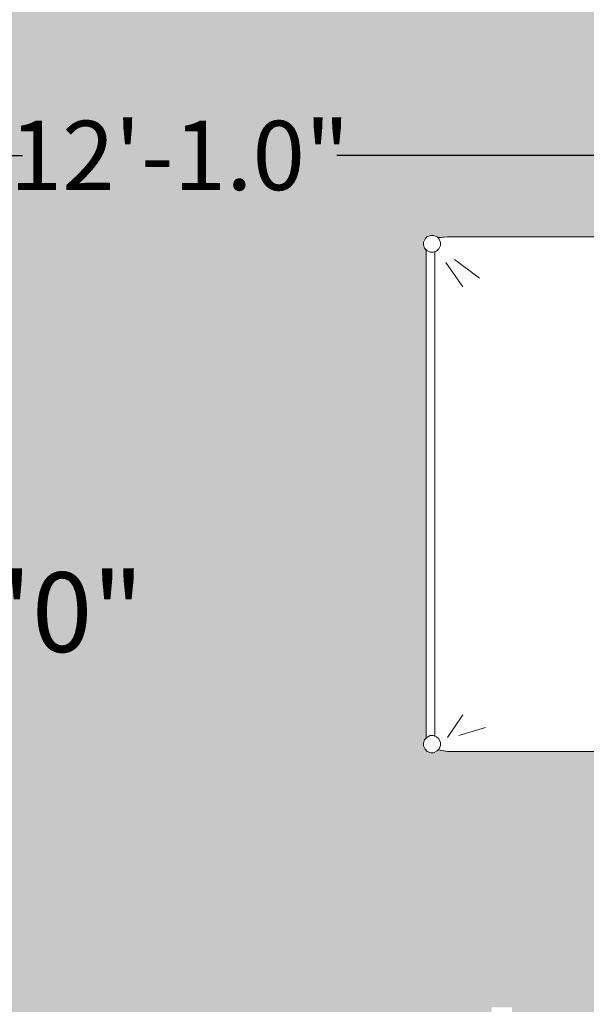
# Model space of a CAD drawing. Units: inches. Extents: x 528 to 2620, y -1066 to 798.
# Tile 8 of 41: x 688 to 737, y 620 to 705. Entities that reach past the tile are written whole.
import ezdxf

# ---------------------------------------------------------------- set-up
doc = ezdxf.new("R2010")
doc.units = ezdxf.units.IN
doc.header["$MEASUREMENT"] = 0
for name, color, linetype, lineweight in [('A-ANNO-DIMS', 2, 'Continuous', 18), ('A-AREA-IDEN', 7, 'Continuous', 18), ('A-FURN', 30, 'Continuous', 18), ('A-WALL-PATT', 8, 'Continuous', 13)]:
    doc.layers.add(name, color=color, linetype=linetype, lineweight=lineweight)
doc.styles.get("Standard").update_dxf_attribs({"font": 'arial.ttf'})
doc.dimstyles.get("Standard").update_dxf_attribs({"dimtxt": 6, "dimasz": 2, "dimexe": 0.18, "dimexo": 0.0625, "dimgap": 0.09, "dimtad": 0, "dimtih": 1, "dimtoh": 1, "dimdec": 1, "dimzin": 0, "dimdsep": 46, "dimlunit": 3, "dimtxsty": 'Standard', "dimblk": 'ARCHTICK', "dimcen": 0.09, "dimadec": 0, "dimazin": 0, "dimtfac": 1, "dimtdec": 1, "dimtofl": 0, "dimtmove": 0, "dimatfit": 3, "dimfxl": 1, "dimtolj": 1, "dimtzin": 0, "dimarcsym": 0})

# ---------------------------------------------------------------- blocks, each defined once
blk = doc.blocks.new('d-bed-3')
at = {"color": 0, "linetype": 'ByBlock'}
for p, q in [((0, 0), (0, -0.5)), ((0.7, 0), (0, 0)), ((0.7, -0.5), (0.7, 0)), ((0.7817, -0.0054), (0.7857, 0.0078)), ((0.7817, -0.0054), (0.7857, 0.0078)), ((0.7857, 0.0078), (0.7968, 0.0166)), ((0.7857, 0.0078), (0.7968, 0.0166)), ((0.7968, 0.0166), (0.8078, 0.0211)), ((0.7968, 0.0166), (0.8078, 0.0211)), ((0.8078, 0.0211), (0.8209, 0.0211)), ((0.8078, 0.0211), (0.8209, 0.0211)), ((0.8209, 0.0211), (0.8349, 0.0144)), ((0.8209, 0.0211), (0.8349, 0.0144)), ((0.8349, 0.0144), (0.8409, 0.0078)), ((0.8349, 0.0144), (0.8429, 0.0056)), ((0.8389, 0.0078), (2.7305, 0.0078)), ((0.8409, 0.0078), (2.7305, 0.0078)), ((0.8429, 0.0056), (0.848, -0.0077)), ((2.7234, -0.0077), (2.7284, 0.0056)), ((2.7284, 0.0056), (2.7365, 0.0144)), ((2.7305, 0.0078), (2.7365, 0.0144)), ((2.7365, 0.0144), (2.7505, 0.0211)), ((2.7365, 0.0144), (2.7505, 0.0211)), ((2.7505, 0.0211), (2.7636, 0.0211)), ((2.7505, 0.0211), (2.7636, 0.0211)), ((2.7636, 0.0211), (2.7746, 0.0166)), ((2.7636, 0.0211), (2.7746, 0.0166)), ((2.7746, 0.0166), (2.7857, 0.0078)), ((2.7746, 0.0166), (2.7857, 0.0078)), ((2.7857, 0.0078), (2.7897, -0.0054)), ((2.7857, 0.0078), (2.7897, -0.0054)), ((2.8714, -0.5), (2.8714, 0)), ((2.8714, 0), (3.5714, 0)), ((3.5714, 0), (3.5714, -0.5)), ((0.7817, -0.0187), (0.7817, -0.0054)), ((0.7817, -0.0187), (0.7817, -0.0054)), ((0.7857, -0.0297), (0.7817, -0.0187)), ((0.7857, -0.0297), (0.7817, -0.0187)), ((0.7857, -2.0939), (0.7857, -0.0297)), ((0.7948, -0.0408), (0.7857, -0.0297)), ((0.7857, -0.032), (0.7857, -2.0939)), ((0.8409, -0.032), (0.8319, -0.0408)), ((0.848, -0.0209), (0.8409, -0.032)), ((0.848, -0.0077), (0.848, -0.0209)), ((2.7234, -0.0209), (2.7234, -0.0077)), ((2.7305, -0.032), (2.7234, -0.0209)), ((2.7395, -0.0408), (2.7305, -0.032)), ((2.7857, -0.0297), (2.7766, -0.0408)), ((2.7857, -0.0297), (2.7766, -0.0408)), ((2.7897, -0.0187), (2.7857, -0.0297)), ((2.7897, -0.0187), (2.7857, -0.0297)), ((2.7897, -0.0054), (2.7897, -0.0187)), ((2.7897, -0.0054), (2.7897, -0.0187)), ((0.05, -0.05), (0.05, -0.45)), ((0.65, -0.05), (0.05, -0.05)), ((0.35, -0.0576), (0.35, -0.4424)), ((0.65, -0.45), (0.65, -0.05)), ((0.8058, -0.0452), (0.7948, -0.0408)), ((0.8188, -0.0452), (0.8058, -0.0452)), ((0.8319, -0.0408), (0.8188, -0.0452)), ((2.7525, -0.0452), (0.8188, -0.0452)), ((2.7525, -0.0452), (2.7395, -0.0408)), ((2.7656, -0.0452), (2.7525, -0.0452)), ((2.7766, -0.0408), (2.7656, -0.0452)), ((2.7766, -0.0408), (2.7656, -0.0452)), ((2.7656, -0.0452), (2.7857, -0.0452)), ((2.7857, -0.0452), (2.7656, -0.0452)), ((2.7857, -2.0939), (2.7857, -0.0452)), ((2.9214, -0.45), (2.9214, -0.05)), ((2.9214, -0.05), (3.5214, -0.05)), ((3.2214, -0.0576), (3.2214, -0.4424)), ((3.5214, -0.05), (3.5214, -0.45)), ((0.8781, -0.1325), (0.8911, -0.1059)), ((0.8911, -0.1059), (0.9182, -0.1082)), ((0.9182, -0.1082), (0.9443, -0.1148)), ((1.0317, -0.117), (1.0588, -0.1082)), ((1.0588, -0.1082), (1.0849, -0.1059)), ((1.0849, -0.1059), (1.113, -0.1104)), ((1.113, -0.1104), (1.1401, -0.117)), ((1.2295, -0.117), (1.2566, -0.1082)), ((1.2566, -0.1082), (1.2827, -0.1059)), ((1.2827, -0.1059), (1.3108, -0.1104)), ((1.3108, -0.1104), (1.3379, -0.117)), ((1.4253, -0.117), (1.4514, -0.1082)), ((1.4514, -0.1082), (1.4805, -0.1059)), ((1.4805, -0.1059), (1.5086, -0.1104)), ((1.5086, -0.1104), (1.5357, -0.117)), ((1.623, -0.1148), (1.6471, -0.1082)), ((1.6471, -0.1082), (1.6763, -0.1059)), ((1.6763, -0.1059), (1.7084, -0.1059)), ((1.7084, -0.1059), (1.7194, -0.1325)), ((1.8489, -0.1302), (1.863, -0.1059)), ((1.863, -0.1059), (1.8951, -0.1059)), ((1.8951, -0.1059), (1.9222, -0.1059)), ((1.9222, -0.1059), (1.9483, -0.1148)), ((2.0357, -0.1148), (2.0628, -0.1082)), ((2.0628, -0.1082), (2.0909, -0.1059)), ((2.0909, -0.1059), (2.117, -0.1082)), ((2.117, -0.1082), (2.1441, -0.1148)), ((2.2335, -0.1148), (2.2606, -0.1082)), ((2.2606, -0.1082), (2.2867, -0.1059)), ((2.2867, -0.1059), (2.3148, -0.1082)), ((2.3148, -0.1082), (2.3419, -0.1148)), ((2.4293, -0.1148), (2.4554, -0.1082)), ((2.4554, -0.1082), (2.4845, -0.1059)), ((2.4845, -0.1059), (2.5126, -0.1082)), ((2.5126, -0.1082), (2.5397, -0.1148)), ((2.627, -0.1148), (2.6511, -0.1059)), ((2.6511, -0.1059), (2.6803, -0.1059)), ((2.6803, -0.1059), (2.6913, -0.1302)), ((0.8721, -0.159), (0.8781, -0.1325)), ((0.9072, -0.5753), (0.9072, -0.1391)), ((0.9072, -0.1391), (1.6763, -0.1391)), ((0.9293, -0.1435), (0.9775, -0.1612)), ((0.9443, -0.1148), (0.9684, -0.128)), ((0.9684, -0.128), (1.0056, -0.128)), ((1.0056, -0.128), (1.0317, -0.117)), ((1.1401, -0.117), (1.1662, -0.128)), ((1.1662, -0.128), (1.2034, -0.128)), ((1.2034, -0.128), (1.2295, -0.117)), ((1.3379, -0.117), (1.362, -0.128)), ((1.362, -0.128), (1.4012, -0.128)), ((1.4012, -0.128), (1.4253, -0.117)), ((1.5357, -0.117), (1.5598, -0.128)), ((1.5598, -0.128), (1.5989, -0.128)), ((1.5989, -0.128), (1.623, -0.1148)), ((1.6471, -0.1501), (1.5989, -0.1656)), ((1.6763, -0.1391), (1.6763, -0.4936)), ((1.7194, -0.1325), (1.7265, -0.159)), ((1.8429, -0.159), (1.8489, -0.1302)), ((2.6622, -0.1369), (1.8931, -0.1369)), ((1.8931, -0.1369), (1.8931, -0.5046)), ((1.9222, -0.1479), (1.9704, -0.1656)), ((1.9483, -0.1148), (1.9724, -0.128)), ((1.9724, -0.128), (2.0096, -0.128)), ((2.0096, -0.128), (2.0357, -0.1148)), ((2.1441, -0.1148), (2.1702, -0.128)), ((2.1702, -0.128), (2.2074, -0.128)), ((2.2074, -0.128), (2.2335, -0.1148)), ((2.3419, -0.1148), (2.366, -0.128)), ((2.366, -0.128), (2.4052, -0.128)), ((2.4052, -0.128), (2.4293, -0.1148)), ((2.5397, -0.1148), (2.5638, -0.128)), ((2.5638, -0.128), (2.6029, -0.128)), ((2.6401, -0.1435), (2.5919, -0.159)), ((2.6029, -0.128), (2.627, -0.1148)), ((2.6622, -0.5753), (2.6622, -0.1369)), ((2.6913, -0.1302), (2.6973, -0.159)), ((0.8741, -0.1866), (0.8721, -0.159)), ((0.8831, -0.2131), (0.8741, -0.1866)), ((0.9223, -0.1612), (0.9333, -0.2042)), ((1.6542, -0.1656), (1.6431, -0.2087)), ((1.7265, -0.1866), (1.7174, -0.2131)), ((1.7265, -0.159), (1.7265, -0.1866)), ((1.8449, -0.1866), (1.8429, -0.159)), ((1.854, -0.2131), (1.8449, -0.1866)), ((1.9152, -0.1656), (1.9263, -0.2087)), ((2.6471, -0.159), (2.6361, -0.202)), ((2.6973, -0.1866), (2.6883, -0.2131)), ((2.6973, -0.159), (2.6973, -0.1866)), ((0.8962, -0.2374), (0.8831, -0.2131)), ((1.7174, -0.2131), (1.7024, -0.2374)), ((1.867, -0.2374), (1.854, -0.2131)), ((2.6883, -0.2131), (2.6732, -0.2374)), ((0.1576, -0.25), (0.5424, -0.25)), ((0.8962, -0.2992), (0.8962, -0.2374)), ((1.7024, -0.2374), (1.7024, -0.2992)), ((1.867, -0.297), (1.867, -0.2374)), ((2.6732, -0.2374), (2.6732, -0.297)), ((3.4138, -0.25), (3.029, -0.25)), ((0.8831, -0.3235), (0.8962, -0.2992)), ((1.7024, -0.2992), (1.7174, -0.3235)), ((1.854, -0.3213), (1.867, -0.297)), ((2.6732, -0.297), (2.6883, -0.3213)), ((0.8761, -0.3489), (0.8831, -0.3235)), ((1.0538, -0.6294), (1.362, -0.3081)), ((1.362, -0.3081), (1.619, -0.5532)), ((1.7174, -0.3235), (1.7244, -0.3489)), ((1.8469, -0.3489), (1.854, -0.3213)), ((2.2074, -0.3081), (1.9483, -0.5532)), ((2.5146, -0.6294), (2.2074, -0.3081)), ((2.6883, -0.3213), (2.6953, -0.3489)), ((0.8761, -0.3776), (0.8761, -0.3489)), ((0.8831, -0.4041), (0.8761, -0.3776)), ((1.3289, -0.3511), (1.3068, -0.3909)), ((1.4052, -0.3467), (1.4122, -0.4019)), ((1.7244, -0.3776), (1.7174, -0.4041)), ((1.7244, -0.3489), (1.7244, -0.3776)), ((1.8469, -0.3754), (1.8469, -0.3489)), ((1.854, -0.4041), (1.8469, -0.3754)), ((2.1632, -0.3445), (2.1572, -0.3997)), ((2.2405, -0.3511), (2.2626, -0.3887)), ((2.6953, -0.3754), (2.6883, -0.4041)), ((2.6953, -0.3489), (2.6953, -0.3754)), ((0.8962, -0.4284), (0.8831, -0.4041)), ((1.3068, -0.3909), (1.3349, -0.4174)), ((1.4122, -0.4019), (1.3901, -0.4284)), ((1.4674, -0.7134), (1.7746, -0.3909)), ((1.7174, -0.4041), (1.7024, -0.4284)), ((1.7746, -0.3909), (2.0979, -0.6979)), ((1.867, -0.4284), (1.854, -0.4041)), ((2.1572, -0.3997), (2.1793, -0.4284)), ((2.2626, -0.3887), (2.2335, -0.4174)), ((2.6883, -0.4041), (2.6732, -0.4284)), ((0.05, -0.45), (0.65, -0.45)), ((0.8962, -0.4781), (0.8962, -0.4284)), ((1.5006, -0.4505), (1.4604, -0.4715)), ((1.7024, -0.4284), (1.7024, -0.4649)), ((1.7415, -0.4351), (1.7194, -0.4737)), ((1.8188, -0.4306), (1.8228, -0.4848)), ((1.867, -0.4781), (1.867, -0.4284)), ((2.0688, -0.4505), (2.109, -0.4715)), ((2.6732, -0.4284), (2.6732, -0.4759)), ((3.5214, -0.45), (2.9214, -0.45)), ((0.8831, -0.5024), (0.8962, -0.4781)), ((1.2255, -0.4715), (1.2626, -0.5223)), ((1.5327, -0.4715), (1.4674, -0.5267)), ((1.7194, -0.4737), (1.7485, -0.5002)), ((1.8228, -0.4848), (1.8008, -0.5113)), ((2.0357, -0.4715), (2.102, -0.5267)), ((2.3439, -0.4715), (2.3068, -0.5201)), ((2.6732, -0.4759), (2.6883, -0.5002)), ((0, -0.5), (0.7, -0.5)), ((0.8721, -0.5576), (0.8741, -0.5289)), ((0.8741, -0.5289), (0.8831, -0.5024)), ((0.9223, -0.5532), (0.9333, -0.5113)), ((1.9112, -0.5333), (1.874, -0.5554)), ((2.6471, -0.5532), (2.6361, -0.5091)), ((2.6883, -0.5002), (2.6973, -0.5267)), ((2.6973, -0.5267), (2.6973, -0.5554)), ((3.5714, -0.5), (2.8714, -0.5)), ((0.8781, -0.5841), (0.8721, -0.5576)), ((0.9293, -0.5709), (0.9775, -0.5532)), ((1.2957, -0.5819), (1.2737, -0.5488)), ((1.3399, -0.5643), (1.3399, -0.5488)), ((1.357, -0.625), (1.3399, -0.5643)), ((1.5989, -0.5488), (1.614, -0.5554)), ((1.6381, -0.5554), (1.6763, -0.6051)), ((1.9443, -0.5554), (1.8781, -0.6096)), ((1.9704, -0.5466), (1.9503, -0.5554)), ((2.2124, -0.6228), (2.2295, -0.5643)), ((2.2295, -0.5643), (2.2295, -0.5466)), ((2.2736, -0.5797), (2.2957, -0.5466)), ((2.6401, -0.5687), (2.5919, -0.5532)), ((2.6973, -0.5554), (2.6913, -0.5841)), ((0.8911, -0.6096), (0.8781, -0.5841)), ((0.9182, -0.6073), (0.8911, -0.6096)), ((1.109, -0.5753), (0.9072, -0.5753)), ((0.9443, -0.6007), (0.9182, -0.6073)), ((0.9684, -0.5886), (0.9443, -0.6007)), ((1.0056, -0.5886), (0.9684, -0.5886)), ((1.0317, -0.5996), (1.0056, -0.5886)), ((1.0588, -0.6073), (1.0317, -0.5996)), ((1.0759, -0.6096), (1.0588, -0.6073)), ((1.105, -0.5864), (1.1271, -0.5864)), ((1.1271, -0.5864), (1.1482, -0.5974)), ((1.1482, -0.5974), (1.1311, -0.5864)), ((1.1311, -0.5864), (1.1592, -0.593)), ((1.3459, -0.625), (1.2957, -0.5819)), ((1.5658, -0.5753), (1.5377, -0.5864)), ((1.5969, -0.5753), (1.5658, -0.5753)), ((1.9684, -0.5753), (2.0036, -0.5753)), ((2.0036, -0.5753), (2.0317, -0.5864)), ((2.1963, -0.6294), (2.124, -0.6118)), ((2.2224, -0.6228), (2.2736, -0.5797)), ((2.4383, -0.5864), (2.4092, -0.5908)), ((2.4423, -0.5864), (2.4202, -0.5974)), ((2.4202, -0.5974), (2.4383, -0.5864)), ((2.4644, -0.5864), (2.4423, -0.5864)), ((2.4604, -0.5753), (2.6622, -0.5753)), ((2.5126, -0.6051), (2.4955, -0.6073)), ((2.5397, -0.5996), (2.5126, -0.6051)), ((2.5638, -0.5864), (2.5397, -0.5996)), ((2.6029, -0.5864), (2.5638, -0.5864)), ((2.627, -0.5996), (2.6029, -0.5864)), ((2.6511, -0.6073), (2.627, -0.5996)), ((2.6803, -0.6073), (2.6511, -0.6073)), ((2.6913, -0.5841), (2.6803, -0.6073)), ((1.3791, -0.9365), (1.0538, -0.6294)), ((1.3138, -0.6626), (1.351, -0.6361)), ((1.368, -0.6626), (1.357, -0.625)), ((1.3731, -0.6294), (1.4453, -0.614)), ((1.3791, -0.6471), (1.4453, -0.6913)), ((1.7084, -0.6648), (1.6873, -0.6316)), ((1.7526, -0.6493), (1.7526, -0.6316)), ((1.7706, -0.7089), (1.7526, -0.6493)), ((2.0387, -0.6427), (2.0427, -0.6405)), ((2.1903, -0.6449), (2.124, -0.6891)), ((2.1903, -0.9365), (2.5146, -0.6294)), ((2.2013, -0.6626), (2.2124, -0.6228)), ((2.2556, -0.6626), (2.2184, -0.6338)), ((1.105, -0.6692), (1.1421, -0.6846)), ((1.1421, -0.6846), (1.1642, -0.6736)), ((1.1642, -0.6736), (1.1753, -0.6692)), ((1.3731, -0.6692), (1.3841, -0.7067)), ((1.7596, -0.7089), (1.7084, -0.6648)), ((1.9765, -0.6604), (1.9503, -0.6714)), ((2.0166, -0.6604), (1.9765, -0.6604)), ((2.0387, -0.6714), (2.0166, -0.6604)), ((2.1963, -0.667), (2.1853, -0.7067)), ((2.4052, -0.6736), (2.3941, -0.667)), ((2.4272, -0.6846), (2.4052, -0.6736)), ((2.4644, -0.667), (2.4272, -0.6846)), ((1.2255, -0.7785), (1.2737, -0.7244)), ((1.4674, -0.7134), (1.4604, -0.7067)), ((1.7897, -1.0193), (1.4674, -0.7134)), ((1.7265, -0.7454), (1.7636, -0.72)), ((1.7817, -0.7454), (1.7706, -0.7089)), ((1.7857, -0.7134), (1.856, -0.6979)), ((2.0979, -0.6979), (1.7897, -1.0193)), ((1.9724, -0.741), (1.9393, -0.7244)), ((2.0538, -0.7609), (2.109, -0.7067)), ((2.3439, -0.7763), (2.2957, -0.7222)), ((1.5548, -0.7675), (1.5397, -0.7631)), ((1.5548, -0.7675), (1.5769, -0.7564)), ((1.5769, -0.7564), (1.5879, -0.752)), ((1.7857, -0.752), (1.7967, -0.7896)), ((1.7897, -0.731), (1.856, -0.7741)), ((2.0096, -0.741), (1.9724, -0.741)), ((2.0497, -0.731), (2.0096, -0.741)), ((1.3791, -0.9365), (1.5357, -0.7763)), ((1.9283, -0.8448), (1.874, -0.7896)), ((2.1903, -0.9365), (2.0277, -0.7697)), ((0.7857, -0.9607), (1.2295, -0.8072)), ((0.9504, -1.2611), (1.5708, -0.8183)), ((1.3178, -0.8382), (1.3239, -0.8117)), ((1.3178, -0.8602), (1.3178, -0.8382)), ((1.4052, -0.8337), (1.4012, -0.8337)), ((1.4052, -0.8768), (1.4052, -0.8337)), ((1.6381, -0.8625), (1.6873, -0.8072)), ((2.618, -1.2611), (1.9855, -0.8161)), ((2.1632, -0.8757), (2.1632, -0.8315)), ((2.1632, -0.8315), (2.1682, -0.8315)), ((2.2515, -0.8382), (2.2445, -0.8094)), ((2.2515, -0.8602), (2.2515, -0.8382)), ((2.7827, -0.9607), (2.3278, -0.8072)), ((1.3349, -0.8879), (1.3178, -0.8602)), ((1.3901, -0.8989), (1.4052, -0.8768)), ((2.1793, -0.8967), (2.1632, -0.8757)), ((2.2335, -0.8856), (2.2515, -0.8602)), ((0.8781, -1.2059), (1.3349, -0.9055)), ((1.7305, -0.921), (1.7375, -0.8945)), ((1.8188, -0.9166), (1.8118, -0.9166)), ((1.8188, -0.9607), (1.8188, -0.9166)), ((2.6913, -1.2059), (2.2254, -0.9055)), ((1.7305, -0.9431), (1.7305, -0.921)), ((1.7485, -0.9718), (1.7305, -0.9431)), ((0.8128, -1.0115), (0.7857, -0.9607)), ((1.8008, -0.9828), (1.8188, -0.9607)), ((2.7676, -0.9895), (2.7455, -1.0259)), ((2.7786, -0.9828), (2.7676, -0.9895)), ((2.7827, -0.9607), (2.7786, -0.9828)), ((0.8128, -1.0325), (0.8128, -1.0115)), ((0.8239, -1.0414), (0.8128, -1.0325)), ((2.7455, -1.0259), (2.7234, -1.0811)), ((0.8299, -1.0635), (0.8239, -1.0414)), ((0.8349, -1.0745), (0.8299, -1.0635)), ((0.845, -1.1032), (0.8349, -1.0745)), ((0.852, -1.1187), (0.845, -1.1032)), ((2.7234, -1.1076), (2.7174, -1.1187)), ((2.7234, -1.0811), (2.7234, -1.1076)), ((0.852, -1.1363), (0.852, -1.1187)), ((0.863, -1.1617), (0.852, -1.1363)), ((2.7124, -1.1253), (2.6953, -1.1617)), ((2.7174, -1.1187), (2.7124, -1.1253)), ((0.867, -1.1905), (0.863, -1.1617)), ((0.9223, -1.2015), (0.9112, -1.1838)), ((2.6582, -1.1838), (2.6471, -1.2015)), ((2.6953, -1.1617), (2.6913, -1.2059)), ((0.8741, -1.1949), (0.867, -1.1905)), ((0.8781, -1.2059), (0.8741, -1.1949)), ((0.9293, -1.2059), (0.9223, -1.2015)), ((0.9403, -1.2236), (0.9293, -1.2059)), ((0.9443, -1.2391), (0.9403, -1.2236)), ((2.6361, -1.2236), (2.625, -1.2391)), ((2.6471, -1.2015), (2.6361, -1.2236)), ((0.9504, -1.2611), (0.9443, -1.2391)), ((2.625, -1.2391), (2.618, -1.2611)), ((2.7234, -2.0497), (2.6913, -1.947)), ((0.8741, -2.0673), (0.9464, -1.9691)), ((0.8851, -2.1005), (0.9795, -2.0342)), ((2.7305, -2.0939), (2.6421, -2.0342)), ((0.7888, -2.1317), (0.7857, -2.0939)), ((0.7857, -2.0939), (0.7887, -2.1303)), ((2.7857, -2.0939), (2.7783, -2.1299)), ((2.7786, -2.1281), (2.7857, -2.0939)), ((0.7797, -2.148), (0.7857, -2.1347)), ((0.7797, -2.148), (0.7857, -2.1347)), ((0.7857, -2.1347), (0.7948, -2.1259)), ((0.7857, -2.1347), (0.7888, -2.1317)), ((0.7948, -2.1259), (0.8078, -2.1215)), ((0.8078, -2.1215), (0.8188, -2.1215)), ((0.8188, -2.1215), (0.8319, -2.1281)), ((0.8319, -2.1281), (0.8409, -2.1369)), ((0.8409, -2.1369), (0.845, -2.1502)), ((2.7284, -2.1369), (2.7234, -2.1502)), ((2.7365, -2.1281), (2.7284, -2.1369)), ((2.7505, -2.1215), (2.7365, -2.1281)), ((2.7616, -2.1215), (2.7505, -2.1215)), ((2.7746, -2.1259), (2.7616, -2.1215)), ((2.7827, -2.1347), (2.7746, -2.1259)), ((2.7783, -2.1299), (2.7827, -2.1347)), ((2.7827, -2.1347), (2.7897, -2.148)), ((2.7897, -2.148), (2.7827, -2.1347)), ((0.7797, -2.159), (0.7797, -2.148)), ((0.7797, -2.148), (0.7797, -2.159)), ((0.7837, -2.1723), (0.7797, -2.159)), ((0.7837, -2.1723), (0.7797, -2.159)), ((0.7927, -2.1811), (0.7837, -2.1723)), ((0.7927, -2.1811), (0.7837, -2.1723)), ((0.8389, -2.1745), (0.8299, -2.1833)), ((0.8367, -2.1767), (0.8299, -2.1833)), ((2.7327, -2.1767), (0.8367, -2.1767)), ((0.845, -2.1612), (0.8389, -2.1745)), ((0.8389, -2.1767), (2.7305, -2.1767)), ((2.7264, -2.1436), (0.845, -2.1436)), ((0.845, -2.1502), (0.845, -2.1612)), ((2.7234, -2.1502), (2.7234, -2.1612)), ((2.7234, -2.1612), (2.7305, -2.1745)), ((2.7305, -2.1745), (2.7395, -2.1833)), ((2.7395, -2.1833), (2.7327, -2.1767)), ((2.7857, -2.1723), (2.7766, -2.1811)), ((2.7766, -2.1811), (2.7857, -2.1723)), ((2.7897, -2.159), (2.7857, -2.1723)), ((2.7857, -2.1723), (2.7897, -2.159)), ((2.7897, -2.148), (2.7897, -2.159)), ((2.7897, -2.159), (2.7897, -2.148)), ((0.8058, -2.1877), (0.7927, -2.1811)), ((0.8058, -2.1877), (0.7927, -2.1811)), ((0.8168, -2.1877), (0.8058, -2.1877)), ((0.8168, -2.1877), (0.8058, -2.1877)), ((0.8299, -2.1833), (0.8168, -2.1877)), ((0.8299, -2.1833), (0.8168, -2.1877)), ((2.7525, -2.1877), (2.7395, -2.1833)), ((2.7395, -2.1833), (2.7525, -2.1877)), ((2.7636, -2.1877), (2.7525, -2.1877)), ((2.7525, -2.1877), (2.7636, -2.1877)), ((2.7766, -2.1811), (2.7636, -2.1877)), ((2.7636, -2.1877), (2.7766, -2.1811))]:
    blk.add_line(p, q, dxfattribs=at)
blk.add_ellipse((0.35, -0.25), major_axis=(-0.1007, 0.1007), ratio=1, dxfattribs=at)
at = {"color": 0, "linetype": 'ByBlock', "extrusion": (0, 0, -1)}
blk.add_ellipse((3.2214, -0.25), major_axis=(0.1007, 0.1007), ratio=1, dxfattribs=at)
blk = doc.blocks.new('_ArchTick')
at = {"color": 0, "linetype": 'ByBlock', "const_width": 0.15}
blk.add_lwpolyline([(-0.5, -0.5), (0.5, 0.5)], dxfattribs=at)
blk = doc.blocks.new('*D25')
at = {"layer": 'A-ANNO-DIMS', "color": 0, "lineweight": -2, "transparency": 16777216}
for p, q in [((629.059, 693.763), (629.059, 693.001)), ((774.059, 693.763), (774.059, 693.001)), ((629.059, 693.181), (687.951, 693.181)), ((774.059, 693.181), (715.168, 693.181))]:
    blk.add_line(p, q, dxfattribs=at)
at = {"layer": 'Defpoints', "color": 0, "transparency": 16777216}
for p in [(629.059, 693.826), (774.059, 693.826), (774.059, 693.181)]:
    blk.add_point(p, dxfattribs=at)
at = {"layer": 'A-ANNO-DIMS', "color": 0, "lineweight": -2, "transparency": 16777216, "xscale": 2, "yscale": 2, "zscale": 2, "rotation": 180}
blk.add_blockref('_ArchTick', (629.059, 693.181), dxfattribs=at)
at = {"layer": 'A-ANNO-DIMS', "color": 0, "lineweight": -2, "transparency": 16777216, "xscale": 2, "yscale": 2, "zscale": 2}
blk.add_blockref('_ArchTick', (774.059, 693.181), dxfattribs=at)
at = {"layer": 'A-ANNO-DIMS', "color": 0, "transparency": 16777216, "insert": (701.559, 693.181), "char_height": 6, "attachment_point": 5}
blk.add_mtext('\\A1;12\'-1.0"', dxfattribs=at)

msp = doc.modelspace()

# ---------------------------------------------------------------- hatches: boundary and pattern name
at = {"layer": 'A-WALL-PATT', "transparency": 33554687}
h = msp.add_hatch(color=256, dxfattribs=at)
h.dxf.hatch_style = 1
h.paths.add_polyline_path([(861.059, 273.922), (817.059, 273.922), (817.059, 272.922), (861.059, 272.922)])
h.paths.add_polyline_path([(817.059, 277.922), (815.059, 277.922), (815.059, 268.922), (817.059, 268.922)])
h.paths.add_polyline_path([(908.059, 397.922), (899.059, 397.922), (899.059, 395.922), (908.059, 395.922)])
h.paths.add_polyline_path([(908.059, 443.922), (899.059, 443.922), (899.059, 441.922), (908.059, 441.922)])
h.paths.add_polyline_path([(904.059, 441.922), (903.059, 441.922), (903.059, 397.922), (904.059, 397.922)])
h.paths.add_polyline_path([(625.059, 561.422), (624.059, 561.422), (624.059, 537.422), (625.059, 537.422)])
h.paths.add_polyline_path([(648.747, 334.444), (720.045, 334.444), (720.045, 344.998), (648.747, 344.998)], flags=9)
h.paths.add_polyline_path([(819.733, 323.153), (880.328, 323.153), (880.328, 333.708), (819.733, 333.708)], flags=9)
h.paths.add_polyline_path([(779.898, 680.607), (821.764, 680.607), (821.764, 691.169), (779.898, 691.169)], flags=9)
h.paths.add_polyline_path([(779.876, 692.362), (817.138, 692.362), (817.138, 703.058), (779.876, 703.058)], flags=9)
h.paths.add_polyline_path([(799.994, 453.884), (860.589, 453.884), (860.589, 464.439), (799.994, 464.439)], flags=9)
h.paths.add_polyline_path([(650.866, 539.397), (708.781, 539.397), (708.781, 549.952), (650.866, 549.952)], flags=9)
h.paths.add_polyline_path([(788.504, 612.01), (849.099, 612.01), (849.099, 622.565), (788.504, 622.565)], flags=9)
h.paths.add_polyline_path([(639.539, 648.31), (700.134, 648.31), (700.134, 658.865), (639.539, 658.865)], flags=9)
h.paths.add_polyline_path([(648.913, 346.09), (747.706, 346.09), (747.706, 356.778), (648.913, 356.778)], flags=9)
h.paths.add_polyline_path([(676.857, 450.66), (746.735, 450.66), (746.735, 461.355), (676.857, 461.355)], flags=9)
h.paths.add_polyline_path([(819.711, 334.947), (865.526, 334.947), (865.526, 345.636), (819.711, 345.636)], flags=9)
h.paths.add_polyline_path([(806.298, 467.745), (874.047, 467.745), (874.047, 478.441), (806.298, 478.441)], flags=9)
h.paths.add_polyline_path([(653.235, 552.284), (690.497, 552.284), (690.497, 562.979), (653.235, 562.979)], flags=9)
h.paths.add_polyline_path([(789.903, 623.407), (843.208, 623.407), (843.208, 634.103), (789.903, 634.103)], flags=9)
h.paths.add_polyline_path([(639.773, 662.103), (693.077, 662.103), (693.077, 672.798), (639.773, 672.798)], flags=9)
h.paths.add_polyline_path([(801.587, 242.914), (846.334, 242.914), (846.334, 253.603), (801.587, 253.603)], flags=9)
h.paths.add_polyline_path([(925.362, 593.982), (925.362, 674.057), (914.673, 674.057), (914.673, 593.982)], flags=9)
h.paths.add_polyline_path([(612.559, 593.982), (612.559, 674.057), (601.871, 674.057), (601.871, 593.982)], flags=9)
h.paths.add_polyline_path([(723.31, 726.564), (803.385, 726.564), (803.385, 737.252), (723.31, 737.252)], flags=9)
at = {"layer": 'A-WALL-PATT', "transparency": 33554590}
h = msp.add_hatch(color=256, dxfattribs=at)
h.dxf.hatch_style = 1
h.paths.add_polyline_path([(774.059, 709.922), (629.059, 709.922), (629.059, 577.922), (728.559, 577.922), (728.559, 579.422), (728.559, 619.422), (730.309, 619.422), (730.309, 619.384, -0.401453), (768.559, 579.422), (768.559, 577.922), (774.059, 577.922)])
h.paths.add_polyline_path([(723.896, 686.058), (723.968, 686.064), (723.828, 686.128)], flags=0)
h.paths.add_polyline_path([(722.785, 642.699), (722.893, 642.756), (722.893, 684.992), (722.647, 685.244), (722.647, 685.82), (723.079, 686.262), (723.533, 686.262), (723.968, 686.064), (724.739, 686.128), (770.696, 686.128), (770.78, 686.14), (771.126, 686.266), (771.694, 686.094), (771.94, 685.478), (771.67, 684.904), (771.582, 684.871), (771.582, 642.782), (771.878, 642.514), (771.878, 641.921), (771.511, 641.462), (770.855, 641.462), (770.401, 641.833), (770.401, 641.551), (724.739, 641.551), (723.991, 641.705), (723.443, 641.414), (722.879, 641.585), (722.597, 642.142)], flags=16)
h.paths.add_polyline_path([(723.994, 641.704), (723.994, 641.707), (723.991, 641.705)], flags=0)
h.paths.add_polyline_path([(722.893, 642.732), (722.893, 684.992), (722.647, 685.244), (722.647, 685.82), (723.079, 686.262), (723.287, 686.262), (722.991, 686.172), (722.794, 685.971), (722.647, 685.68), (722.647, 685.434), (722.745, 685.143), (722.942, 684.942), (723.238, 684.807), (723.484, 684.807), (723.779, 684.897), (723.976, 685.098), (724.174, 685.488), (724.124, 685.635), (724.124, 685.249), (723.631, 684.746), (723.631, 642.961), (724.124, 642.514), (724.124, 641.887), (723.656, 641.462), (723.079, 641.462), (722.647, 641.904), (722.647, 642.48)], flags=0)
h.paths.add_polyline_path([(722.647, 642.29), (722.647, 642.044), (722.794, 641.753), (723.079, 641.462), (723.287, 641.462), (722.879, 641.585), (722.597, 642.142)], flags=0)
h.paths.add_polyline_path([(770.745, 686.128), (770.58, 686.128), (770.551, 686.057)], flags=0)
h.paths.add_polyline_path([(743.299, 645.288), (753.227, 659.398), (748.69, 663.75), (753.234, 668.538), (743.299, 682.458), (743.791, 682.592), (744.136, 682.681), (744.53, 682.928), (744.628, 683.084), (745.017, 683.327), (744.53, 684.069), (744.776, 684.158), (744.874, 684.315), (745.514, 684.404), (746.081, 684.651), (746.474, 684.651), (746.819, 684.807), (747.459, 685.031), (747.705, 685.143), (748.198, 685.277), (748.394, 685.523), (748.862, 685.523), (749.994, 686.128), (753.488, 676.03), (757.379, 680.153), (757.791, 679.758), (758.044, 680.645), (758.29, 681.227), (758.29, 682.055), (758.019, 682.592), (757.871, 683.174), (757.822, 683.778), (758.388, 684.069), (758.979, 684.203), (759.619, 684.158), (760.21, 683.957), (760.751, 683.666), (761.859, 683.666), (762.401, 683.957), (762.991, 684.114), (763.631, 684.114), (764.198, 683.957), (764.739, 683.666), (766.118, 683.666), (766.659, 683.957), (767.25, 684.158), (767.865, 684.203), (768.456, 684.069), (769.047, 683.778), (768.998, 683.174), (768.85, 682.592), (768.554, 682.055), (768.554, 681.227), (768.801, 680.645), (769.092, 679.75), (768.948, 678.832), (768.801, 678.228), (768.554, 677.646), (768.554, 676.818), (768.801, 676.237), (769.092, 675.341), (768.948, 674.424), (768.801, 673.82), (768.554, 673.283), (768.554, 672.41), (768.801, 671.873), (768.998, 671.291), (769.047, 670.642), (768.948, 670.016), (768.801, 669.411), (768.554, 668.874), (768.554, 668.002), (768.974, 667.239), (769.047, 666.279), (769.047, 665.563), (768.456, 665.316), (767.865, 665.16), (767.25, 665.16), (766.659, 665.361), (766.118, 665.697), (764.739, 665.697), (763.945, 665.204), (762.991, 665.204), (762.401, 665.361), (761.859, 665.697), (761.005, 665.697), (762.696, 664.086), (760.741, 662.027), (761.859, 662.027), (762.401, 662.318), (763.342, 662.548), (764.247, 662.318), (764.788, 662.027), (766.118, 662.027), (766.659, 662.318), (767.25, 662.519), (767.865, 662.564), (768.505, 662.43), (769.047, 662.116), (769.047, 661.4), (769.047, 660.796), (768.85, 660.214), (768.554, 659.677), (768.554, 658.849), (768.85, 658.267), (768.998, 657.663), (769.069, 656.749), (768.85, 655.851), (768.554, 655.269), (768.554, 654.441), (768.85, 653.859), (769.069, 652.961), (768.998, 652.046), (768.85, 651.442), (768.554, 650.905), (768.554, 650.032), (768.85, 649.495), (768.998, 648.914), (769.047, 648.265), (768.998, 647.638), (768.85, 647.034), (768.554, 646.497), (768.554, 645.624), (768.85, 645.087), (769.047, 644.55), (769.047, 643.901), (768.505, 643.655), (767.865, 643.521), (767.25, 643.521), (766.659, 643.722), (766.118, 644.058), (764.788, 644.058), (764.247, 643.722), (763.342, 643.492), (762.401, 643.722), (761.859, 644.058), (760.801, 644.058), (760.259, 643.722), (759.668, 643.521), (759.028, 643.521), (758.388, 643.655), (757.871, 643.901), (757.871, 644.55), (758.044, 645.087), (758.339, 645.624), (758.339, 646.497), (758.044, 647.034), (757.921, 647.638), (757.866, 648.059), (757.379, 647.593), (753.422, 651.773), (749.994, 641.618), (749.502, 641.708), (749.354, 641.954), (748.542, 642.446), (747.311, 642.939), (746.652, 642.939), (746.327, 643.185), (745.514, 643.565), (744.53, 643.655), (745.011, 644.4), (744.628, 644.639), (744.136, 644.886), (743.791, 645.132)], flags=0)
h.paths.add_polyline_path([(755.656, 654.933), (756.542, 654.687), (757.527, 654.329), (756.641, 654.575)], flags=0)
h.paths.add_polyline_path([(758.339, 649.204), (758.339, 648.712), (758.585, 644.304), (758.585, 648.802)], flags=0)
h.paths.add_polyline_path([(758.339, 649.294), (758.093, 649.697), (758.359, 649.165)], flags=0)
h.paths.add_polyline_path([(755.656, 672.79), (756.493, 673.037), (757.358, 673.351), (757.353, 673.358), (756.641, 673.149)], flags=0)
h.paths.add_polyline_path([(760.264, 639.641), (771.408, 639.641), (771.408, 624.039), (760.264, 624.039)], flags=16)
h.paths.add_polyline_path([(761.378, 638.526), (770.294, 638.526), (770.294, 625.153), (761.378, 625.153)], flags=0)
edge = h.paths.add_edge_path(flags=0)
edge.add_ellipse((765.836, 631.84), major_axis=(-2.245, 2.245), ratio=1, start_angle=-45, end_angle=45, ccw=False)
edge.add_ellipse((765.836, 631.84), major_axis=(-2.245, 2.245), ratio=1, start_angle=-135, end_angle=-45, ccw=False)
edge.add_ellipse((765.836, 631.84), major_axis=(-2.245, 2.245), ratio=1, start_angle=135, end_angle=-135, ccw=False)
edge.add_ellipse((765.836, 631.84), major_axis=(-2.245, 2.245), ratio=1, start_angle=45, end_angle=135, ccw=False)
h.paths.add_polyline_path([(758.585, 683.42), (758.585, 678.922), (758.373, 678.575), (758.339, 678.43), (758.093, 678.049), (758.339, 678.519), (758.339, 679.011)], flags=0)
h.paths.add_polyline_path([(760.264, 688.038), (760.264, 703.64), (771.408, 703.64), (771.408, 688.038)], flags=16)
h.paths.add_polyline_path([(770.401, 685.389), (770.401, 685.846), (770.855, 686.217), (771.511, 686.217), (771.878, 685.758), (771.878, 685.165), (771.582, 684.897), (771.582, 642.782), (771.878, 642.514), (771.878, 641.921), (771.511, 641.462), (770.855, 641.462), (770.401, 641.833), (770.401, 642.29)], flags=0)
h.paths.add_polyline_path([(770.532, 642.678), (771.052, 643.009), (771.67, 642.775), (771.94, 642.201), (771.694, 641.585), (771.126, 641.413), (770.551, 641.622), (770.347, 642.132)], flags=16)
h.paths.add_polyline_path([(761.378, 689.152), (761.378, 702.526), (770.294, 702.526), (770.294, 689.152)], flags=0)
edge = h.paths.add_edge_path(flags=0)
edge.add_ellipse((765.836, 695.839), major_axis=(2.245, 2.245), ratio=1, start_angle=405, end_angle=495, ccw=False)
edge.add_ellipse((765.836, 695.839), major_axis=(2.245, 2.245), ratio=1, start_angle=675, end_angle=765, ccw=False)
edge.add_ellipse((765.836, 695.839), major_axis=(2.245, 2.245), ratio=1, start_angle=585, end_angle=675, ccw=False)
edge.add_ellipse((765.836, 695.839), major_axis=(2.245, 2.245), ratio=1, start_angle=495, end_angle=585, ccw=False)
h.paths.add_polyline_path([(770.696, 684.897), (770.942, 684.74), (771.41, 684.74), (771.73, 685.031), (771.878, 685.344), (771.878, 685.635), (771.694, 686.094), (771.582, 686.128), (771.878, 685.758), (771.878, 685.165), (771.41, 684.74), (770.849, 684.74)], flags=0)
h.paths.add_polyline_path([(899.059, 709.922), (831.059, 709.922), (831.059, 699.922), (829.809, 699.922), (829.809, 675.922), (831.059, 675.922), (831.059, 669.422), (778.559, 669.422), (778.559, 567.172), (780.059, 567.172), (820.059, 567.172), (820.059, 565.422), (820.021, 565.422, -0.401453), (780.059, 527.172), (778.559, 527.172), (778.559, 525.422), (899.059, 525.422)])
h.paths.add_polyline_path([(849.197, 636.014), (849.269, 636.02), (849.129, 636.084)], flags=0)
h.paths.add_polyline_path([(848.193, 634.948), (847.947, 635.2), (847.947, 635.776), (848.379, 636.218), (848.833, 636.218), (849.269, 636.02), (850.039, 636.084), (895.996, 636.084), (896.081, 636.096), (896.426, 636.222), (896.995, 636.05), (897.241, 635.434), (896.97, 634.86), (896.883, 634.827), (896.883, 592.738), (897.178, 592.47), (897.178, 591.877), (896.811, 591.418), (896.155, 591.418), (895.701, 591.789), (895.701, 591.507), (850.039, 591.507), (849.292, 591.661), (848.744, 591.37), (848.18, 591.541), (847.897, 592.098), (848.086, 592.655), (848.193, 592.712)], flags=16)
h.paths.add_polyline_path([(849.294, 591.66), (849.295, 591.663), (849.292, 591.661)], flags=16)
h.paths.add_polyline_path([(848.193, 634.948), (847.947, 635.2), (847.947, 635.776), (848.379, 636.218), (848.587, 636.218), (848.292, 636.128), (848.095, 635.927), (847.947, 635.636), (847.947, 635.39), (848.046, 635.099), (848.243, 634.897), (848.538, 634.763), (848.784, 634.763), (849.079, 634.853), (849.276, 635.054), (849.474, 635.444), (849.424, 635.591), (849.424, 635.205), (848.932, 634.702), (848.932, 592.917), (849.424, 592.47), (849.424, 591.843), (848.956, 591.418), (848.379, 591.418), (847.947, 591.86), (847.947, 592.436), (848.193, 592.688)], flags=0)
h.paths.add_polyline_path([(847.947, 592.246), (847.947, 592), (848.095, 591.709), (848.379, 591.418), (848.587, 591.418), (848.18, 591.541), (847.897, 592.098)], flags=16)
h.paths.add_polyline_path([(896.046, 636.084), (895.88, 636.084), (895.852, 636.013)], flags=0)
h.paths.add_polyline_path([(868.599, 632.414), (869.092, 632.548), (869.436, 632.637), (869.83, 632.884), (869.929, 633.04), (870.318, 633.283), (869.83, 634.025), (870.076, 634.114), (870.175, 634.271), (870.815, 634.36), (871.381, 634.607), (871.775, 634.607), (872.119, 634.763), (872.759, 634.987), (873.006, 635.099), (873.498, 635.233), (873.695, 635.479), (874.163, 635.479), (875.295, 636.084), (878.788, 625.986), (882.679, 630.109), (883.091, 629.714), (883.344, 630.601), (883.59, 631.183), (883.59, 632.011), (883.319, 632.548), (883.172, 633.13), (883.123, 633.734), (883.689, 634.025), (884.279, 634.159), (884.919, 634.114), (885.51, 633.913), (886.052, 633.622), (887.159, 633.622), (887.701, 633.913), (888.292, 634.07), (888.932, 634.07), (889.498, 633.913), (890.039, 633.622), (891.418, 633.622), (891.959, 633.913), (892.55, 634.114), (893.166, 634.159), (893.756, 634.025), (894.347, 633.734), (894.298, 633.13), (894.15, 632.548), (893.855, 632.011), (893.855, 631.183), (894.101, 630.601), (894.393, 629.706), (894.249, 628.788), (894.101, 628.184), (893.855, 627.602), (893.855, 626.774), (894.101, 626.193), (894.393, 625.297), (894.249, 624.38), (894.101, 623.776), (893.855, 623.239), (893.855, 622.366), (894.101, 621.829), (894.298, 621.247), (894.347, 620.598), (894.249, 619.972), (894.101, 619.367), (893.855, 618.83), (893.855, 617.958), (894.274, 617.195), (894.347, 616.235), (894.347, 615.518), (893.756, 615.272), (893.166, 615.116), (892.55, 615.116), (891.959, 615.317), (891.418, 615.653), (890.039, 615.653), (889.245, 615.16), (888.292, 615.16), (887.701, 615.317), (887.159, 615.653), (886.305, 615.653), (887.996, 614.042), (886.041, 611.983), (887.159, 611.983), (887.701, 612.274), (888.642, 612.504), (889.547, 612.274), (890.089, 611.983), (891.418, 611.983), (891.959, 612.274), (892.55, 612.475), (893.166, 612.52), (893.806, 612.386), (894.347, 612.072), (894.347, 611.356), (894.347, 610.752), (894.15, 610.17), (893.855, 609.633), (893.855, 608.805), (894.15, 608.223), (894.298, 607.619), (894.37, 606.705), (894.15, 605.807), (893.855, 605.225), (893.855, 604.397), (894.15, 603.815), (894.37, 602.917), (894.298, 602.002), (894.15, 601.398), (893.855, 600.861), (893.855, 599.988), (894.15, 599.451), (894.298, 598.87), (894.347, 598.221), (894.298, 597.594), (894.15, 596.99), (893.855, 596.453), (893.855, 595.58), (894.15, 595.043), (894.347, 594.506), (894.347, 593.857), (893.806, 593.611), (893.166, 593.477), (892.55, 593.477), (891.959, 593.678), (891.418, 594.014), (890.089, 594.014), (889.547, 593.678), (888.642, 593.448), (887.701, 593.678), (887.159, 594.014), (886.101, 594.014), (885.559, 593.678), (884.969, 593.477), (884.329, 593.477), (883.689, 593.611), (883.172, 593.857), (883.172, 594.506), (883.344, 595.043), (883.639, 595.58), (883.639, 596.453), (883.344, 596.99), (883.221, 597.594), (883.167, 598.015), (882.679, 597.549), (878.722, 601.729), (875.295, 591.574), (874.803, 591.664), (874.655, 591.91), (873.843, 592.402), (872.612, 592.895), (871.952, 592.895), (871.627, 593.141), (870.815, 593.521), (869.83, 593.611), (870.311, 594.356), (869.929, 594.595), (869.436, 594.842), (869.092, 595.088), (868.599, 595.244), (878.528, 609.354), (873.99, 613.706), (878.535, 618.494)], flags=0)
h.paths.add_polyline_path([(880.956, 622.746), (881.793, 622.993), (882.659, 623.307), (882.654, 623.314), (881.941, 623.104)], flags=0)
h.paths.add_polyline_path([(880.956, 604.889), (881.843, 604.643), (882.827, 604.285), (881.941, 604.531)], flags=16)
h.paths.add_polyline_path([(883.393, 628.005), (883.639, 628.475), (883.639, 628.967), (883.886, 633.376), (883.886, 628.878), (883.674, 628.531), (883.639, 628.386)], flags=0)
h.paths.add_polyline_path([(883.639, 599.16), (883.639, 598.668), (883.886, 594.26), (883.886, 598.758)], flags=16)
h.paths.add_polyline_path([(883.639, 599.25), (883.393, 599.653), (883.659, 599.121)], flags=16)
h.paths.add_polyline_path([(885.564, 637.994), (885.564, 653.596), (896.709, 653.596), (896.709, 637.994)], flags=16)
h.paths.add_polyline_path([(885.564, 589.597), (896.709, 589.597), (896.709, 573.995), (885.564, 573.995)], flags=16)
h.paths.add_polyline_path([(886.679, 639.108), (886.679, 652.482), (895.594, 652.482), (895.594, 639.108)], flags=0)
h.paths.add_polyline_path([(886.679, 588.482), (895.594, 588.482), (895.594, 575.109), (886.679, 575.109)], flags=0)
edge = h.paths.add_edge_path(flags=0)
edge.add_ellipse((891.136, 645.795), major_axis=(2.245, 2.245), ratio=1, start_angle=405, end_angle=495, ccw=False)
edge.add_ellipse((891.136, 645.795), major_axis=(2.245, 2.245), ratio=1, start_angle=675, end_angle=765, ccw=False)
edge.add_ellipse((891.136, 645.795), major_axis=(2.245, 2.245), ratio=1, start_angle=585, end_angle=675, ccw=False)
edge.add_ellipse((891.136, 645.795), major_axis=(2.245, 2.245), ratio=1, start_angle=495, end_angle=585, ccw=False)
edge = h.paths.add_edge_path(flags=0)
edge.add_ellipse((891.136, 581.796), major_axis=(-2.245, 2.245), ratio=1, start_angle=-45, end_angle=45, ccw=False)
edge.add_ellipse((891.136, 581.796), major_axis=(-2.245, 2.245), ratio=1, start_angle=-135, end_angle=-45, ccw=False)
edge.add_ellipse((891.136, 581.796), major_axis=(-2.245, 2.245), ratio=1, start_angle=135, end_angle=-135, ccw=False)
edge.add_ellipse((891.136, 581.796), major_axis=(-2.245, 2.245), ratio=1, start_angle=45, end_angle=135, ccw=False)
h.paths.add_polyline_path([(895.701, 635.345), (895.701, 635.802), (896.155, 636.173), (896.811, 636.173), (897.178, 635.714), (897.178, 635.121), (896.883, 634.853), (896.883, 592.738), (897.178, 592.47), (897.178, 591.877), (896.811, 591.418), (896.155, 591.418), (895.701, 591.789), (895.701, 592.246)], flags=0)
h.paths.add_polyline_path([(895.996, 634.853), (896.243, 634.696), (896.71, 634.696), (897.03, 634.987), (897.178, 635.3), (897.178, 635.591), (896.995, 636.05), (896.883, 636.084), (897.178, 635.714), (897.178, 635.121), (896.71, 634.696), (896.15, 634.696)], flags=0)
h.paths.add_polyline_path([(895.832, 592.634), (896.353, 592.965), (896.97, 592.731), (897.241, 592.157), (896.995, 591.541), (896.426, 591.369), (895.852, 591.578), (895.648, 592.088)], flags=16)
h.paths.add_polyline_path([(725.255, 569.422), (724.059, 569.422), (724.059, 573.422), (629.059, 573.422), (629.059, 525.422), (724.059, 525.422), (724.059, 545.422), (725.255, 545.422)])
h.paths.add_polyline_path([(820.021, 565.422), (780.059, 565.422), (780.059, 567.172), (774.059, 567.172), (774.059, 567.422), (774.059, 573.422), (768.559, 573.422), (768.481, 577.922), (768.559, 577.922), (768.559, 579.422, 0.401453), (730.309, 619.384), (730.309, 579.422), (728.559, 579.422), (728.559, 573.422), (728.559, 569.422), (727.255, 569.422), (727.255, 545.422), (728.559, 545.422), (728.559, 520.922), (665.059, 520.922), (665.059, 436.422), (716.059, 436.422), (716.059, 421.422), (717.809, 421.422), (717.809, 421.358, -0.392996), (740.059, 397.422, -0.392996), (762.309, 421.358), (762.309, 421.422), (764.059, 421.422), (764.059, 400.422), (770.059, 400.422), (779.059, 400.422), (779.059, 391.422), (779.059, 359.767), (795.432, 359.767), (795.432, 294.295), (893.669, 294.295), (893.669, 277.922), (899.059, 277.922), (899.059, 391.422), (851.059, 391.422), (851.059, 395.922), (899.059, 395.922), (899.059, 443.922), (899.059, 520.922), (774.059, 520.922), (774.059, 527.172), (778.559, 527.172), (780.059, 527.172, 0.401453)])
h.paths.add_polyline_path([(774.059, 519.657), (842.122, 519.657), (842.122, 505.072), (788.644, 505.072), (788.644, 474.079), (788.644, 470.433, -0.883215), (779.529, 456.663), (774.971, 456.663, -0.414214), (774.059, 457.575)], flags=16)
h.paths.add_polyline_path([(775.883, 517.834), (840.299, 517.834), (840.299, 514.188), (788.644, 514.188), (788.644, 484.41), (779.529, 484.41), (779.529, 474.079), (775.883, 474.079)], flags=0)
h.paths.add_polyline_path([(706.7, 501.564, -0.254069), (706.7, 493.021), (698.31, 492.555), (698.31, 502.031)], flags=16)
h.paths.add_polyline_path([(691.334, 515.692), (691.8, 507.301), (682.325, 507.301), (682.791, 515.692, -0.254069)], flags=16)
h.paths.add_polyline_path([(695.485, 504.685), (695.485, 479.416), (678.64, 479.416), (678.64, 504.685)], flags=16)
h.paths.add_polyline_path([(706.7, 489.602, -0.254069), (706.7, 481.058), (698.31, 480.592), (698.31, 490.068)], flags=16)
h.paths.add_polyline_path([(675.815, 502.031), (675.815, 492.555), (667.425, 493.021, -0.254069), (667.425, 501.564)], flags=16)
h.paths.add_polyline_path([(691.8, 476.8), (691.334, 468.409, -0.254069), (682.791, 468.409), (682.325, 476.8)], flags=16)
h.paths.add_polyline_path([(675.815, 490.068), (675.815, 480.592), (667.425, 481.058, -0.254069), (667.425, 489.602)], flags=16)
h.paths.add_polyline_path([(764.059, 397.422), (762.309, 397.422), (762.309, 421.358, 0.392996), (740.059, 397.422, 0.392996), (717.809, 421.358), (717.809, 397.422), (716.059, 397.422), (716.059, 391.422), (716.059, 385.422), (764.059, 385.422), (764.059, 391.422)], flags=17)
h.paths.add_polyline_path([(716.059, 436.422), (705.859, 436.422), (705.859, 418.422), (716.059, 418.422), (716.059, 421.422)], flags=17)
h.paths.add_polyline_path([(716.059, 418.422), (705.859, 418.422), (705.859, 400.422), (716.059, 400.422)], flags=17)
h.paths.add_polyline_path([(705.859, 418.422), (695.659, 418.422), (695.659, 400.422), (696.559, 400.422), (705.859, 400.422)], flags=17)
h.paths.add_polyline_path([(705.859, 436.422), (695.659, 436.422), (695.659, 418.422), (705.859, 418.422)], flags=17)
h.paths.add_polyline_path([(695.659, 418.422), (685.459, 418.422), (685.459, 400.422), (695.659, 400.422)], flags=17)
h.paths.add_polyline_path([(695.659, 436.422), (685.459, 436.422), (685.459, 418.422), (695.659, 418.422)], flags=17)
h.paths.add_polyline_path([(685.459, 418.422), (675.259, 418.422), (675.259, 400.422), (685.459, 400.422)], flags=17)
h.paths.add_polyline_path([(685.459, 436.422), (675.259, 436.422), (675.259, 418.422), (685.459, 418.422)], flags=17)
h.paths.add_polyline_path([(675.259, 436.422), (665.059, 436.422), (665.059, 418.422), (675.259, 418.422)])
h.paths.add_polyline_path([(675.259, 418.422), (665.059, 418.422), (665.059, 400.422), (675.259, 400.422)])
h.paths.add_polyline_path([(665.059, 418.422), (646.967, 418.422), (646.991, 436.422), (629.059, 436.422), (629.059, 400.422), (665.059, 400.422)])
h.paths.add_polyline_path([(665.059, 436.422), (646.991, 436.422), (646.967, 418.422), (665.059, 418.422)], flags=17)
h.paths.add_polyline_path([(647.005, 446.622), (629.059, 446.622), (629.059, 436.672), (629.059, 436.422), (646.991, 436.422)])
h.paths.add_polyline_path([(665.059, 446.622), (647.005, 446.622), (646.991, 436.422), (665.059, 436.422)])
h.paths.add_polyline_path([(647.019, 456.822), (629.059, 456.822), (629.059, 446.622), (647.005, 446.622)])
h.paths.add_polyline_path([(665.059, 456.822), (647.019, 456.822), (647.005, 446.622), (665.059, 446.622)])
h.paths.add_polyline_path([(647.032, 467.022), (629.059, 467.022), (629.059, 456.822), (647.019, 456.822)])
h.paths.add_polyline_path([(665.059, 467.022), (647.032, 467.022), (647.019, 456.822), (665.059, 456.822)])
h.paths.add_polyline_path([(665.059, 477.222), (647.046, 477.222), (647.032, 467.022), (665.059, 467.022)])
h.paths.add_polyline_path([(647.046, 477.222), (629.059, 477.222), (629.059, 467.022), (647.032, 467.022)])
h.paths.add_polyline_path([(647.059, 487.222), (629.059, 487.222), (629.059, 477.222), (647.046, 477.222), (647.048, 479.019), (645.53, 483.246), (640.877, 480.371)])
h.paths.add_polyline_path([(665.059, 520.922), (629.059, 520.922), (629.059, 487.222), (647.059, 487.222), (665.059, 487.222)])
h.paths.add_polyline_path([(665.059, 487.222), (647.059, 487.222), (653.224, 480.355), (648.578, 483.242), (647.048, 479.019), (647.046, 477.222), (665.059, 477.222)])

# ---------------------------------------------------------------- block references
at = {"layer": 'A-FURN', "xscale": 22.28859121186505, "yscale": 22.28859121186505, "zscale": 22.28859121186505, "rotation": 270}
msp.add_blockref('d-bed-3', (771.408, 703.64), dxfattribs=at)

# ---------------------------------------------------------------- texts
at = {"layer": 'A-AREA-IDEN'}
msp.add_text('12\' 1" X 11\'0"', height=6.89074, dxfattribs=at).set_placement((641.298, 650.187))

# ---------------------------------------------------------------- dimensions: what is measured, and where the dimension line sits
at = {"layer": 'A-ANNO-DIMS'}
dim = msp.add_linear_dim(base=(774.059, 693.181), p1=(629.059, 693.826), p2=(774.059, 693.826), dimstyle='Standard', override={"dimclrd": 0, "dimclre": 0, "dimclrt": 0}, dxfattribs=at)
dim.commit()
dim.dimension.update_dxf_attribs({"geometry": '*D25', "text_midpoint": (701.559, 693.181)})

doc.saveas('drawing.dxf')
